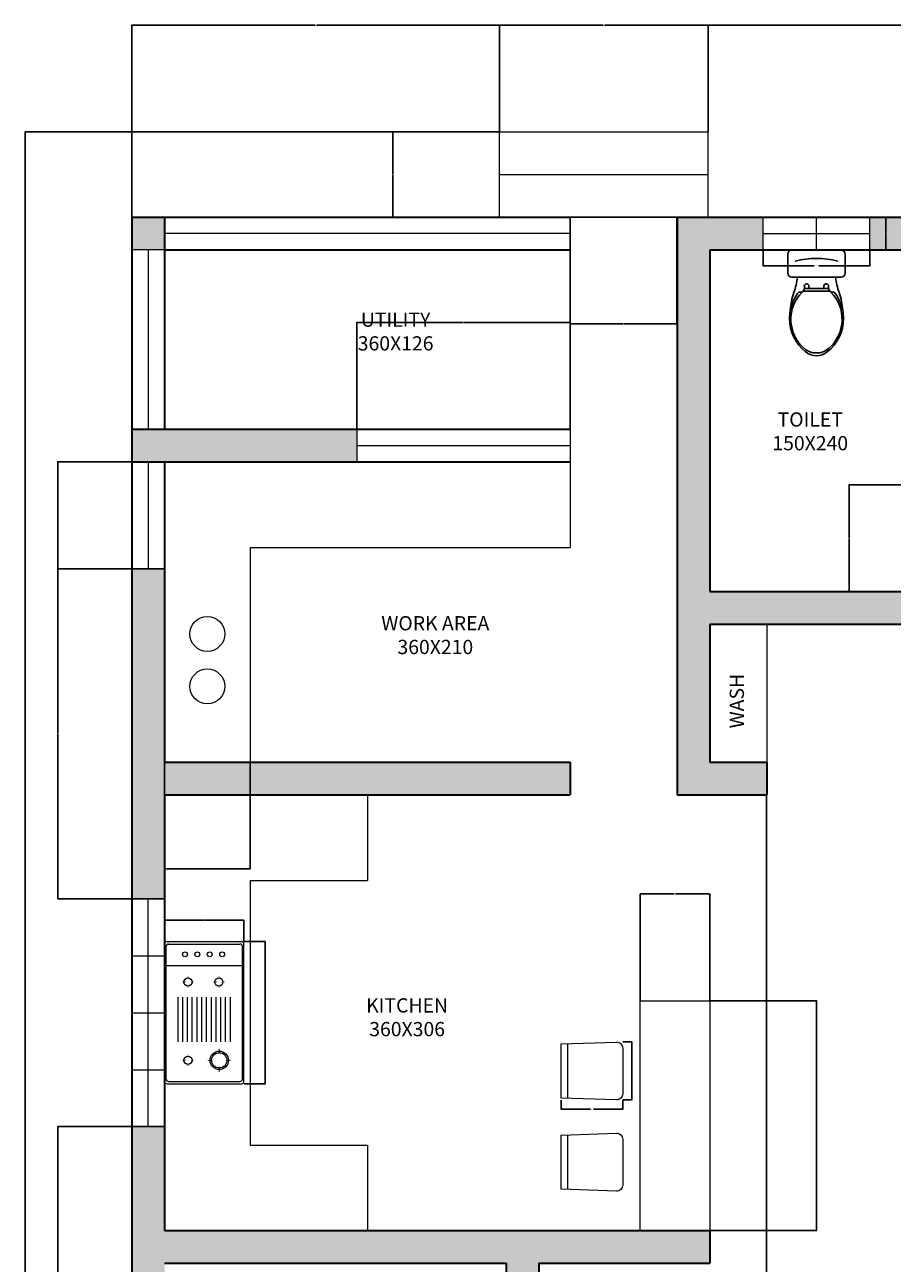
# Model space of a CAD drawing. Units: centimetres. Extents: x 2178 to 3635, y 1064 to 2635.
# Tile 5 of 9: x 2178 to 2788, y 1765 to 2635. Entities that reach past the tile are written whole.
import ezdxf

# ---------------------------------------------------------------- set-up
doc = ezdxf.new("R2010")
doc.units = ezdxf.units.CM
for name, color, linetype, lineweight in [('A-ANNO-DIMS', 2, 'Continuous', 18), ('A-AREA-IDEN', 7, 'Continuous', 18), ('A-DOOR', 32, 'Continuous', 25), ('A-EQPM', 42, 'Continuous', 18), ('A-FLOR-CASE', 32, 'Continuous', 18), ('A-FLOR-FIXT', 42, 'Continuous', 18), ('A-FLOR-STRS', 7, 'Continuous', 18), ('A-FURN', 42, 'Continuous', 18), ('A-GLAZ', 4, 'Continuous', 18), ('A-WALL', 7, 'Continuous', 35)]:
    doc.layers.add(name, color=color, linetype=linetype, lineweight=lineweight)
doc.layers.add('A-WALL-PATT', color=18, linetype='Continuous', lineweight=13, true_color=0x000000)
doc.layers.add('WC-Detail_dwgmodels.com', color=251, linetype='Continuous')
doc.layers.add('WC-Outline_dwgmodels.com', color=250, linetype='Continuous')
doc.styles.get("Standard").update_dxf_attribs({"font": 'arial.ttf'})
doc.dimstyles.get("Standard").update_dxf_attribs({"dimtxt": 0.18, "dimasz": 0.18, "dimexe": 0.18, "dimexo": 0.0625, "dimgap": 0.09, "dimtad": 0, "dimtih": 1, "dimtoh": 1, "dimdec": 4, "dimzin": 0, "dimdsep": 46, "dimtxsty": 'Standard', "dimcen": 0.09, "dimadec": 0, "dimazin": 0, "dimtfac": 1, "dimtdec": 4, "dimtofl": 0, "dimtmove": 0, "dimatfit": 3, "dimfxl": 1, "dimtolj": 1, "dimtzin": 0, "dimarcsym": 0})

# ---------------------------------------------------------------- blocks, each defined once
blk = doc.blocks.new('pan')
at = {"layer": 'WC-Detail_dwgmodels.com'}
for p, q in [((2845.06, 2654.5), (2845.98, 2656.18)), ((2854.51, 2654.5), (2845.06, 2654.5)), ((2845.98, 2656.18), (2845.98, 2658.01)), ((2849.25, 2656.18), (2845.98, 2656.18)), ((2849.25, 2658.01), (2849.25, 2656.18)), ((2854.51, 2656.18), (2849.25, 2656.18)), ((2854.51, 2656.18), (2859.76, 2656.18)), ((2854.51, 2654.5), (2863.95, 2654.5)), ((2859.76, 2658.01), (2859.76, 2656.18)), ((2859.76, 2656.18), (2863.04, 2656.18)), ((2863.04, 2656.18), (2863.04, 2658.01)), ((2863.95, 2654.5), (2863.04, 2656.18)), ((2844.36, 2653.82), (2842.09, 2653.82)), ((2864.65, 2653.82), (2866.93, 2653.82))]:
    blk.add_line(p, q, dxfattribs=at)
for centre, radius, start, end in [((2854.54, 2618.37), 59.08, 90.02796, 104.67123), ((2854.48, 2618.37), 59.08, 75.32877, 89.97204), ((2863.72, 2634.72), 27.2, 133.32364, 135.38283), ((2847.61, 2658.01), 1.64, 0, 180), ((2861.4, 2658.01), 1.64, 0, 180), ((2845.29, 2634.72), 27.2, 44.61717, 46.67636), ((2863.72, 2634.72), 27.2, 135.38283, 229.26806), ((2865.36, 2635.16), 29.83, 141.274, 162.76494), ((2845.29, 2634.72), 27.2, 310.73194, 44.61717), ((2843.66, 2635.16), 29.83, 14.64821, 38.726), ((2865.36, 2635.16), 29.83, 162.76494, 168.85834), ((2843.66, 2635.16), 29.83, 11.14166, 14.64821), ((2854.36, 2623.84), 12.85, 229.26806, 270.66836), ((2854.66, 2623.84), 12.85, 269.33164, 310.73194)]:
    blk.add_arc(centre, radius, start, end, dxfattribs=at)
at = {"layer": 'WC-Outline_dwgmodels.com'}
for p, q in [((2834.37, 2680.53), (2834.37, 2667.05)), ((2854.51, 2683.42), (2837.26, 2683.42)), ((2871.75, 2683.42), (2854.51, 2683.42)), ((2874.65, 2667.05), (2874.65, 2680.53)), ((2837.26, 2664.16), (2841.21, 2664.16)), ((2841.21, 2664.16), (2854.51, 2664.16)), ((2867.8, 2664.16), (2854.51, 2664.16)), ((2867.8, 2664.16), (2871.75, 2664.16))]:
    blk.add_line(p, q, dxfattribs=at)
for centre, radius, start, end in [((2837.26, 2680.53), 2.89, 90, 180), ((2871.75, 2680.53), 2.89, 360, 90), ((2837.26, 2667.05), 2.89, 180, 270), ((2788.54, 2671.16), 53.13, 340.44424, 352.4299), ((2920.47, 2671.16), 53.13, 187.5701, 199.55576), ((2871.75, 2667.05), 2.89, 270, 0), ((2880.9, 2638.36), 44.88, 160.44424, 176.71895), ((2828.12, 2638.36), 44.88, 3.28105, 19.55576), ((2865.36, 2635.16), 29.83, 168.85834, 179.8559), ((2843.66, 2635.16), 29.83, 0.1441, 11.14166), ((2865.36, 2635.16), 29.83, 179.8559, 231.74169), ((2843.66, 2635.16), 29.83, 308.25831, 0.1441), ((2854.51, 2621.4), 12.31, 231.74169, 269.98853), ((2854.5, 2621.4), 12.31, 270.01147, 308.25831)]:
    blk.add_arc(centre, radius, start, end, dxfattribs=at)
blk = doc.blocks.new('cooktop')
for p, q in [((2318.02, 2660.21), (2318.02, 2613.21)), ((2319.52, 2661.71), (2406.13, 2661.71)), ((2319.52, 2659.21), (2319.52, 2614.21)), ((2321.02, 2660.71), (2404.63, 2660.71)), ((2392.56, 2660.71), (2392.56, 2612.71)), ((2406.13, 2659.21), (2406.13, 2614.21)), ((2407.63, 2660.21), (2407.63, 2613.21)), ((2332.64, 2648.75), (2333.04, 2648.75)), ((2344.49, 2653.27), (2372.74, 2653.27)), ((2344.49, 2650.27), (2372.74, 2650.27)), ((2344.49, 2647.27), (2372.74, 2647.27)), ((2382.04, 2648.75), (2382.44, 2648.75)), ((2344.49, 2644.27), (2372.74, 2644.27)), ((2344.49, 2641.27), (2372.74, 2641.27)), ((2344.49, 2638.27), (2372.74, 2638.27)), ((2344.49, 2635.27), (2372.74, 2635.27)), ((2344.49, 2632.27), (2372.74, 2632.27)), ((2344.49, 2629.27), (2372.74, 2629.27)), ((2344.49, 2626.27), (2372.74, 2626.27)), ((2344.49, 2623.27), (2372.74, 2623.27)), ((2382.04, 2629.31), (2382.44, 2629.31)), ((2344.49, 2620.27), (2372.74, 2620.27)), ((2319.52, 2611.71), (2406.13, 2611.71)), ((2321.02, 2612.71), (2404.63, 2612.71))]:
    blk.add_line(p, q)
for centre, radius in [((2332.84, 2646.95), 2.58), ((2382.24, 2646.95), 2.58), ((2399.61, 2648.89), 1.53), ((2399.61, 2641.09), 1.53), ((2332.84, 2627.26), 5.81), ((2332.84, 2627.26), 4.81), ((2399.61, 2633.28), 1.53), ((2382.24, 2627.51), 2.58), ((2399.61, 2625.48), 1.53)]:
    blk.add_circle(centre, radius)
for centre, start, end in [((2319.52, 2660.21), 90, 180), ((2321.02, 2659.21), 90, 180), ((2404.63, 2659.21), 0, 90), ((2406.13, 2660.21), 0, 90), ((2319.52, 2613.21), 180, 270), ((2321.02, 2614.21), 180, 270), ((2404.63, 2614.21), 270, 0), ((2406.13, 2613.21), 270, 0)]:
    blk.add_arc(centre, 1.5, start, end)
for points in [[(2329.26, 2646.75), (2329.26, 2647.15), (2331.04, 2646.75), (2331.04, 2647.15)], [(2332.64, 2650.53), (2333.04, 2650.53), (2332.64, 2648.75), (2333.04, 2648.75)], [(2336.42, 2647.15), (2336.42, 2646.75), (2334.64, 2647.15), (2334.64, 2646.75)], [(2378.66, 2646.75), (2378.66, 2647.15), (2380.44, 2646.75), (2380.44, 2647.15)], [(2382.04, 2650.53), (2382.44, 2650.53), (2382.04, 2648.75), (2382.44, 2648.75)], [(2385.82, 2647.15), (2385.82, 2646.75), (2384.04, 2647.15), (2384.04, 2646.75)], [(2333.04, 2643.37), (2332.64, 2643.37), (2333.04, 2645.14), (2332.64, 2645.14)], [(2382.44, 2643.37), (2382.04, 2643.37), (2382.44, 2645.14), (2382.04, 2645.14)], [(2332.54, 2634.56), (2333.14, 2634.56), (2332.54, 2631.56), (2333.14, 2631.56)], [(2382.04, 2631.09), (2382.44, 2631.09), (2382.04, 2629.31), (2382.44, 2629.31)], [(2325.54, 2626.96), (2325.54, 2627.56), (2328.54, 2626.96), (2328.54, 2627.56)], [(2333.14, 2619.95), (2332.54, 2619.95), (2333.14, 2622.96), (2332.54, 2622.96)], [(2340.15, 2627.56), (2340.15, 2626.96), (2337.14, 2627.56), (2337.14, 2626.96)], [(2378.66, 2627.31), (2378.66, 2627.71), (2380.44, 2627.31), (2380.44, 2627.71)], [(2382.44, 2623.93), (2382.04, 2623.93), (2382.44, 2625.71), (2382.04, 2625.71)], [(2385.82, 2627.71), (2385.82, 2627.31), (2384.04, 2627.71), (2384.04, 2627.31)]]:
    blk.add_solid(points)
blk = doc.blocks.new('c')
blk.add_lwpolyline([(3808.85, 1833.77), (3776.18, 1834.86), (3776.18, 1867.04), (3808.85, 1868.12, -0.424007), (3812.61, 1864.48), (3812.61, 1837.41, -0.424007)], format="xyb", close=True)
blk.add_lwpolyline([(3779.83, 1867.16), (3779.83, 1834.74)])
blk = doc.blocks.new('WIN-1600-4LT')
for p, q in [((0, 23), (0, 0)), ((40, 23), (40, 0)), ((80, 23), (80, 0)), ((120, 23), (120, 0)), ((160, 23), (160, 0)), ((0, 11.5), (160, 11.5))]:
    blk.add_line(p, q)
blk = doc.blocks.new('WIN-0750-2LT')
for p, q in [((0, 0), (0, 23)), ((37.5, 0), (37.5, 23)), ((75, 0), (75, 23)), ((0, 11.5), (75, 11.5))]:
    blk.add_line(p, q)
blk = doc.blocks.new('DOOR-0750')
blk.add_line((0, 0), (75, 0))
blk = doc.blocks.new('*D22')
at = {"layer": 'A-ANNO-DIMS', "color": 0, "lineweight": -2, "transparency": 16777216}
for p, q in [((2555.32, 1879.23), (2555.32, 1872.64)), ((2555.5, 1872.82), (2575.93, 1872.82)), ((2598.28, 1872.82), (2577.84, 1872.82)), ((2598.46, 1879.23), (2598.46, 1872.64))]:
    blk.add_line(p, q, dxfattribs=at)
at = {"layer": 'A-ANNO-DIMS', "color": 0, "transparency": 16777216}
for points in [[(2555.5, 1872.85), (2555.5, 1872.79), (2555.32, 1872.82)], [(2598.28, 1872.85), (2598.28, 1872.79), (2598.46, 1872.82)]]:
    blk.add_solid(points, dxfattribs=at)
at = {"layer": 'Defpoints', "color": 0, "transparency": 16777216}
for p in [(2555.32, 1879.29), (2598.46, 1879.29), (2598.46, 1872.82)]:
    blk.add_point(p, dxfattribs=at)
at = {"layer": 'A-ANNO-DIMS', "color": 0, "transparency": 16777216, "insert": (2576.89, 1872.82), "char_height": 0.18, "attachment_point": 5}
blk.add_mtext('\\A1;CHAIR 43 TYP.', dxfattribs=at)
blk = doc.blocks.new('*D23')
at = {"layer": 'A-ANNO-DIMS', "color": 0, "lineweight": -2, "transparency": 16777216}
for p, q in [((2598.52, 1920.05), (2605.11, 1920.05)), ((2604.93, 1919.87), (2604.93, 1899.85)), ((2604.93, 1879.47), (2604.93, 1899.49)), ((2598.52, 1879.29), (2605.11, 1879.29))]:
    blk.add_line(p, q, dxfattribs=at)
at = {"layer": 'A-ANNO-DIMS', "color": 0, "transparency": 16777216}
for points in [[(2604.9, 1919.87), (2604.96, 1919.87), (2604.93, 1920.05)], [(2604.9, 1879.47), (2604.96, 1879.47), (2604.93, 1879.29)]]:
    blk.add_solid(points, dxfattribs=at)
at = {"layer": 'Defpoints', "color": 0, "transparency": 16777216}
for p in [(2598.46, 1920.05), (2604.93, 1920.05), (2598.46, 1879.29)]:
    blk.add_point(p, dxfattribs=at)
at = {"layer": 'A-ANNO-DIMS', "color": 0, "transparency": 16777216, "insert": (2604.93, 1899.67), "char_height": 0.18, "attachment_point": 5}
blk.add_mtext('\\A1;41 TYP.', dxfattribs=at)
blk = doc.blocks.new('*D32')
at = {"layer": 'A-ANNO-DIMS', "color": 0, "lineweight": -2, "transparency": 16777216}
for p, q in [((2697.1, 2476.53), (2697.1, 2465.16)), ((2772.1, 2476.53), (2772.1, 2465.16)), ((2697.28, 2465.34), (2732.97, 2465.34)), ((2771.92, 2465.34), (2736.24, 2465.34))]:
    blk.add_line(p, q, dxfattribs=at)
at = {"layer": 'A-ANNO-DIMS', "color": 0, "transparency": 16777216}
for points in [[(2697.28, 2465.37), (2697.28, 2465.31), (2697.1, 2465.34)], [(2771.92, 2465.37), (2771.92, 2465.31), (2772.1, 2465.34)]]:
    blk.add_solid(points, dxfattribs=at)
at = {"layer": 'Defpoints', "color": 0, "transparency": 16777216}
for p in [(2697.1, 2476.59), (2772.1, 2476.59), (2772.1, 2465.34)]:
    blk.add_point(p, dxfattribs=at)
at = {"layer": 'A-ANNO-DIMS', "color": 0, "transparency": 16777216, "insert": (2734.6, 2465.34), "char_height": 0.18, "attachment_point": 5}
blk.add_mtext('\\A1;2-LIGHT WINDOW 75 TYP.', dxfattribs=at)
blk = doc.blocks.new('*D33')
at = {"layer": 'A-ANNO-DIMS', "color": 0, "lineweight": -2, "transparency": 16777216}
for p, q in [((2772.17, 2499.59), (2783.53, 2499.59)), ((2783.35, 2499.41), (2783.35, 2488.27)), ((2783.35, 2476.77), (2783.35, 2487.91)), ((2772.17, 2476.59), (2783.53, 2476.59))]:
    blk.add_line(p, q, dxfattribs=at)
at = {"layer": 'A-ANNO-DIMS', "color": 0, "transparency": 16777216}
for points in [[(2783.32, 2499.41), (2783.38, 2499.41), (2783.35, 2499.59)], [(2783.32, 2476.77), (2783.38, 2476.77), (2783.35, 2476.59)]]:
    blk.add_solid(points, dxfattribs=at)
at = {"layer": 'Defpoints', "color": 0, "transparency": 16777216}
for p in [(2772.1, 2499.59), (2783.35, 2499.59), (2772.1, 2476.59)]:
    blk.add_point(p, dxfattribs=at)
at = {"layer": 'A-ANNO-DIMS', "color": 0, "transparency": 16777216, "insert": (2783.35, 2488.09), "char_height": 0.18, "attachment_point": 5}
blk.add_mtext('\\A1;23 TYP.', dxfattribs=at)
blk = doc.blocks.new('*D44')
at = {"layer": 'A-ANNO-DIMS', "color": 0, "lineweight": -2, "transparency": 16777216}
for p, q in [((2332.41, 1990.54), (2347.51, 1990.54)), ((2347.33, 1990.36), (2347.33, 1940.77)), ((2347.33, 1890.82), (2347.33, 1940.41)), ((2332.41, 1890.64), (2347.51, 1890.64))]:
    blk.add_line(p, q, dxfattribs=at)
at = {"layer": 'A-ANNO-DIMS', "color": 0, "transparency": 16777216}
for points in [[(2347.3, 1990.36), (2347.36, 1990.36), (2347.33, 1990.54)], [(2347.3, 1890.82), (2347.36, 1890.82), (2347.33, 1890.64)]]:
    blk.add_solid(points, dxfattribs=at)
at = {"layer": 'Defpoints', "color": 0, "transparency": 16777216}
for p in [(2332.35, 1990.54), (2347.33, 1990.54), (2332.35, 1890.64)]:
    blk.add_point(p, dxfattribs=at)
at = {"layer": 'A-ANNO-DIMS', "color": 0, "transparency": 16777216, "insert": (2347.33, 1940.59), "char_height": 0.18, "attachment_point": 5}
blk.add_mtext('\\A1;COOKTOP 100', dxfattribs=at)
blk = doc.blocks.new('*D45')
at = {"layer": 'A-ANNO-DIMS', "color": 0, "lineweight": -2, "transparency": 16777216}
for p, q in [((2276.6, 1990.6), (2276.6, 2005.7)), ((2276.78, 2005.52), (2304.26, 2005.52)), ((2332.17, 2005.52), (2304.69, 2005.52)), ((2332.35, 1990.6), (2332.35, 2005.7))]:
    blk.add_line(p, q, dxfattribs=at)
at = {"layer": 'A-ANNO-DIMS', "color": 0, "transparency": 16777216}
for points in [[(2276.78, 2005.55), (2276.78, 2005.49), (2276.6, 2005.52)], [(2332.17, 2005.55), (2332.17, 2005.49), (2332.35, 2005.52)]]:
    blk.add_solid(points, dxfattribs=at)
at = {"layer": 'Defpoints', "color": 0, "transparency": 16777216}
for p in [(2276.6, 2005.52), (2276.6, 1990.54), (2332.35, 1990.54)]:
    blk.add_point(p, dxfattribs=at)
at = {"layer": 'A-ANNO-DIMS', "color": 0, "transparency": 16777216, "insert": (2304.47, 2005.52), "char_height": 0.18, "attachment_point": 5}
blk.add_mtext('\\A1;56', dxfattribs=at)
blk = doc.blocks.new('*D47')
at = {"layer": 'A-ANNO-DIMS', "color": 0, "lineweight": -2, "transparency": 16777216}
for p, q in [((2511.88, 2559.59), (2178.42, 2559.59)), ((2178.6, 2559.41), (2178.6, 1874.27)), ((2178.6, 1188.77), (2178.6, 1873.91)), ((2253.54, 1188.59), (2178.42, 1188.59))]:
    blk.add_line(p, q, dxfattribs=at)
at = {"layer": 'A-ANNO-DIMS', "color": 0, "transparency": 16777216}
for points in [[(2178.57, 2559.41), (2178.63, 2559.41), (2178.6, 2559.59)], [(2178.57, 1188.77), (2178.63, 1188.77), (2178.6, 1188.59)]]:
    blk.add_solid(points, dxfattribs=at)
at = {"layer": 'Defpoints', "color": 0, "transparency": 16777216}
for p in [(2178.6, 2559.59), (2511.95, 2559.59), (2253.6, 1188.59)]:
    blk.add_point(p, dxfattribs=at)
at = {"layer": 'A-ANNO-DIMS', "color": 0, "transparency": 16777216, "insert": (2178.6, 1874.09), "char_height": 0.18, "attachment_point": 5}
blk.add_mtext('\\A1;1371', dxfattribs=at)
blk = doc.blocks.new('*D48')
at = {"layer": 'A-ANNO-DIMS', "color": 0, "lineweight": -2, "transparency": 16777216}
for p, q in [((2253.6, 2499.65), (2253.6, 2634.77)), ((2253.78, 2634.59), (2382.31, 2634.59)), ((2511.77, 2634.59), (2383.24, 2634.59)), ((2511.95, 2559.65), (2511.95, 2634.77))]:
    blk.add_line(p, q, dxfattribs=at)
at = {"layer": 'A-ANNO-DIMS', "color": 0, "transparency": 16777216}
for points in [[(2253.78, 2634.62), (2253.78, 2634.56), (2253.6, 2634.59)], [(2511.77, 2634.62), (2511.77, 2634.56), (2511.95, 2634.59)]]:
    blk.add_solid(points, dxfattribs=at)
at = {"layer": 'Defpoints', "color": 0, "transparency": 16777216}
for p in [(2511.95, 2634.59), (2511.95, 2559.59), (2253.6, 2499.59)]:
    blk.add_point(p, dxfattribs=at)
at = {"layer": 'A-ANNO-DIMS', "color": 0, "transparency": 16777216, "insert": (2382.78, 2634.59), "char_height": 0.18, "attachment_point": 5}
blk.add_mtext('\\A1;258.34', dxfattribs=at)
blk = doc.blocks.new('*D49')
at = {"layer": 'A-ANNO-DIMS', "color": 0, "lineweight": -2, "transparency": 16777216}
for p, q in [((2511.95, 2559.65), (2511.95, 2634.77)), ((2512.13, 2634.59), (2584.8, 2634.59)), ((2658.38, 2634.59), (2585.71, 2634.59)), ((2658.56, 2559.65), (2658.56, 2634.77))]:
    blk.add_line(p, q, dxfattribs=at)
at = {"layer": 'A-ANNO-DIMS', "color": 0, "transparency": 16777216}
for points in [[(2512.13, 2634.62), (2512.13, 2634.56), (2511.95, 2634.59)], [(2658.38, 2634.62), (2658.38, 2634.56), (2658.56, 2634.59)]]:
    blk.add_solid(points, dxfattribs=at)
at = {"layer": 'Defpoints', "color": 0, "transparency": 16777216}
for p in [(2658.56, 2634.59), (2511.95, 2559.59), (2658.56, 2559.59)]:
    blk.add_point(p, dxfattribs=at)
at = {"layer": 'A-ANNO-DIMS', "color": 0, "transparency": 16777216, "insert": (2585.25, 2634.59), "char_height": 0.18, "attachment_point": 5}
blk.add_mtext('\\A1;146.62', dxfattribs=at)
blk = doc.blocks.new('*D50')
at = {"layer": 'A-ANNO-DIMS', "color": 0, "lineweight": -2, "transparency": 16777216}
for p, q in [((2658.56, 2559.65), (2658.56, 2634.77)), ((2658.74, 2634.59), (2926.79, 2634.59)), ((3195.42, 2634.59), (2927.37, 2634.59)), ((3195.6, 2499.65), (3195.6, 2634.77))]:
    blk.add_line(p, q, dxfattribs=at)
at = {"layer": 'A-ANNO-DIMS', "color": 0, "transparency": 16777216}
for points in [[(2658.74, 2634.62), (2658.74, 2634.56), (2658.56, 2634.59)], [(3195.42, 2634.62), (3195.42, 2634.56), (3195.6, 2634.59)]]:
    blk.add_solid(points, dxfattribs=at)
at = {"layer": 'Defpoints', "color": 0, "transparency": 16777216}
for p in [(3195.6, 2634.59), (2658.56, 2559.59), (3195.6, 2499.59)]:
    blk.add_point(p, dxfattribs=at)
at = {"layer": 'A-ANNO-DIMS', "color": 0, "transparency": 16777216, "insert": (2927.08, 2634.59), "char_height": 0.18, "attachment_point": 5}
blk.add_mtext('\\A1;537', dxfattribs=at)
blk = doc.blocks.new('*D52')
at = {"layer": 'A-ANNO-DIMS', "color": 0, "lineweight": -2, "transparency": 16777216}
for p, q in [((2511.88, 2559.59), (2436.77, 2559.59)), ((2436.95, 2559.41), (2436.95, 2529.77)), ((2436.95, 2499.77), (2436.95, 2529.41)), ((2511.88, 2499.59), (2436.77, 2499.59))]:
    blk.add_line(p, q, dxfattribs=at)
at = {"layer": 'A-ANNO-DIMS', "color": 0, "transparency": 16777216}
for points in [[(2436.92, 2559.41), (2436.98, 2559.41), (2436.95, 2559.59)], [(2436.92, 2499.77), (2436.98, 2499.77), (2436.95, 2499.59)]]:
    blk.add_solid(points, dxfattribs=at)
at = {"layer": 'Defpoints', "color": 0, "transparency": 16777216}
for p in [(2436.95, 2559.59), (2511.95, 2559.59), (2511.95, 2499.59)]:
    blk.add_point(p, dxfattribs=at)
at = {"layer": 'A-ANNO-DIMS', "color": 0, "transparency": 16777216, "insert": (2436.95, 2529.59), "char_height": 0.18, "attachment_point": 5}
blk.add_mtext('\\A1;60', dxfattribs=at)
blk = doc.blocks.new('*D63')
at = {"layer": 'A-ANNO-DIMS', "color": 0, "lineweight": -2, "transparency": 16777216}
for p, q in [((2699.6, 2093.53), (2699.6, 1113.41)), ((2809.6, 2093.53), (2809.6, 1113.41)), ((2699.78, 1113.59), (2754.32, 1113.59)), ((2809.42, 1113.59), (2754.88, 1113.59))]:
    blk.add_line(p, q, dxfattribs=at)
at = {"layer": 'A-ANNO-DIMS', "color": 0, "transparency": 16777216}
for points in [[(2699.78, 1113.62), (2699.78, 1113.56), (2699.6, 1113.59)], [(2809.42, 1113.62), (2809.42, 1113.56), (2809.6, 1113.59)]]:
    blk.add_solid(points, dxfattribs=at)
at = {"layer": 'Defpoints', "color": 0, "transparency": 16777216}
for p in [(2699.6, 2093.59), (2809.6, 2093.59), (2809.6, 1113.59)]:
    blk.add_point(p, dxfattribs=at)
at = {"layer": 'A-ANNO-DIMS', "color": 0, "transparency": 16777216, "insert": (2754.6, 1113.59), "char_height": 0.18, "attachment_point": 5}
blk.add_mtext('\\A1;110', dxfattribs=at)
blk = doc.blocks.new('*D64')
at = {"layer": 'A-ANNO-DIMS', "color": 0, "lineweight": -2, "transparency": 16777216}
for p, q in [((2561.6, 2499.53), (2561.6, 2424.41)), ((2636.6, 2499.53), (2636.6, 2424.41)), ((2561.78, 2424.59), (2598.89, 2424.59)), ((2636.42, 2424.59), (2599.32, 2424.59))]:
    blk.add_line(p, q, dxfattribs=at)
at = {"layer": 'A-ANNO-DIMS', "color": 0, "transparency": 16777216}
for points in [[(2561.78, 2424.62), (2561.78, 2424.56), (2561.6, 2424.59)], [(2636.42, 2424.62), (2636.42, 2424.56), (2636.6, 2424.59)]]:
    blk.add_solid(points, dxfattribs=at)
at = {"layer": 'Defpoints', "color": 0, "transparency": 16777216}
for p in [(2561.6, 2499.59), (2636.6, 2499.59), (2561.6, 2424.59)]:
    blk.add_point(p, dxfattribs=at)
at = {"layer": 'A-ANNO-DIMS', "color": 0, "transparency": 16777216, "insert": (2599.1, 2424.59), "char_height": 0.18, "attachment_point": 5}
blk.add_mtext('\\A1;75', dxfattribs=at)
blk = doc.blocks.new('*D66')
at = {"layer": 'A-ANNO-DIMS', "color": 0, "lineweight": -2, "transparency": 16777216}
for p, q in [((2832.54, 2311.59), (2757.42, 2311.59)), ((2757.6, 2311.41), (2757.6, 2274.27)), ((2757.6, 2236.77), (2757.6, 2273.91)), ((2832.54, 2236.59), (2757.42, 2236.59))]:
    blk.add_line(p, q, dxfattribs=at)
at = {"layer": 'A-ANNO-DIMS', "color": 0, "transparency": 16777216}
for points in [[(2757.57, 2311.41), (2757.63, 2311.41), (2757.6, 2311.59)], [(2757.57, 2236.77), (2757.63, 2236.77), (2757.6, 2236.59)]]:
    blk.add_solid(points, dxfattribs=at)
at = {"layer": 'Defpoints', "color": 0, "transparency": 16777216}
for p in [(2757.6, 2311.59), (2832.6, 2311.59), (2832.6, 2236.59)]:
    blk.add_point(p, dxfattribs=at)
at = {"layer": 'A-ANNO-DIMS', "color": 0, "transparency": 16777216, "insert": (2757.6, 2274.09), "char_height": 0.18, "attachment_point": 5}
blk.add_mtext('\\A1;75', dxfattribs=at)
blk = doc.blocks.new('*D72')
at = {"layer": 'A-ANNO-DIMS', "color": 0, "lineweight": -2, "transparency": 16777216}
for p, q in [((2276.54, 1860.59), (2201.42, 1860.59)), ((2201.6, 1860.41), (2201.6, 1796.52)), ((2201.6, 1732.27), (2201.6, 1796.16)), ((2276.54, 1732.09), (2201.42, 1732.09))]:
    blk.add_line(p, q, dxfattribs=at)
at = {"layer": 'A-ANNO-DIMS', "color": 0, "transparency": 16777216}
for points in [[(2201.57, 1860.41), (2201.63, 1860.41), (2201.6, 1860.59)], [(2201.57, 1732.27), (2201.63, 1732.27), (2201.6, 1732.09)]]:
    blk.add_solid(points, dxfattribs=at)
at = {"layer": 'Defpoints', "color": 0, "transparency": 16777216}
for p in [(2201.6, 1860.59), (2276.6, 1860.59), (2276.6, 1732.09)]:
    blk.add_point(p, dxfattribs=at)
at = {"layer": 'A-ANNO-DIMS', "color": 0, "transparency": 16777216, "insert": (2201.6, 1796.34), "char_height": 0.18, "attachment_point": 5}
blk.add_mtext('\\A1;128.5', dxfattribs=at)
blk = doc.blocks.new('*D73')
at = {"layer": 'A-ANNO-DIMS', "color": 0, "lineweight": -2, "transparency": 16777216}
for p, q in [((2276.54, 2252.59), (2201.42, 2252.59)), ((2201.6, 2252.41), (2201.6, 2136.77)), ((2201.6, 2020.77), (2201.6, 2136.41)), ((2276.54, 2020.59), (2201.42, 2020.59))]:
    blk.add_line(p, q, dxfattribs=at)
at = {"layer": 'A-ANNO-DIMS', "color": 0, "transparency": 16777216}
for points in [[(2201.57, 2252.41), (2201.63, 2252.41), (2201.6, 2252.59)], [(2201.57, 2020.77), (2201.63, 2020.77), (2201.6, 2020.59)]]:
    blk.add_solid(points, dxfattribs=at)
at = {"layer": 'Defpoints', "color": 0, "transparency": 16777216}
for p in [(2201.6, 2252.59), (2276.6, 2252.59), (2276.6, 2020.59)]:
    blk.add_point(p, dxfattribs=at)
at = {"layer": 'A-ANNO-DIMS', "color": 0, "transparency": 16777216, "insert": (2201.6, 2136.59), "char_height": 0.18, "attachment_point": 5}
blk.add_mtext('\\A1;232', dxfattribs=at)
blk = doc.blocks.new('*D74')
at = {"layer": 'A-ANNO-DIMS', "color": 0, "lineweight": -2, "transparency": 16777216}
for p, q in [((2276.54, 2327.59), (2201.42, 2327.59)), ((2201.6, 2327.41), (2201.6, 2290.27)), ((2201.6, 2252.77), (2201.6, 2289.91)), ((2276.54, 2252.59), (2201.42, 2252.59))]:
    blk.add_line(p, q, dxfattribs=at)
at = {"layer": 'A-ANNO-DIMS', "color": 0, "transparency": 16777216}
for points in [[(2201.57, 2327.41), (2201.63, 2327.41), (2201.6, 2327.59)], [(2201.57, 2252.77), (2201.63, 2252.77), (2201.6, 2252.59)]]:
    blk.add_solid(points, dxfattribs=at)
at = {"layer": 'Defpoints', "color": 0, "transparency": 16777216}
for p in [(2201.6, 2327.59), (2276.6, 2327.59), (2276.6, 2252.59)]:
    blk.add_point(p, dxfattribs=at)
at = {"layer": 'A-ANNO-DIMS', "color": 0, "transparency": 16777216, "insert": (2201.6, 2290.09), "char_height": 0.18, "attachment_point": 5}
blk.add_mtext('\\A1;75', dxfattribs=at)
blk = doc.blocks.new('*D81')
at = {"layer": 'A-ANNO-DIMS', "color": 0, "lineweight": -2, "transparency": 16777216}
for p, q in [((2276.6, 2116.53), (2276.6, 2041.41)), ((2336.6, 2116.53), (2336.6, 2041.41)), ((2276.78, 2041.59), (2306.39, 2041.59)), ((2336.42, 2041.59), (2306.82, 2041.59))]:
    blk.add_line(p, q, dxfattribs=at)
at = {"layer": 'A-ANNO-DIMS', "color": 0, "transparency": 16777216}
for points in [[(2276.78, 2041.62), (2276.78, 2041.56), (2276.6, 2041.59)], [(2336.42, 2041.62), (2336.42, 2041.56), (2336.6, 2041.59)]]:
    blk.add_solid(points, dxfattribs=at)
at = {"layer": 'Defpoints', "color": 0, "transparency": 16777216}
for p in [(2276.6, 2116.59), (2336.6, 2116.59), (2276.6, 2041.59)]:
    blk.add_point(p, dxfattribs=at)
at = {"layer": 'A-ANNO-DIMS', "color": 0, "transparency": 16777216, "insert": (2306.6, 2041.59), "char_height": 0.18, "attachment_point": 5}
blk.add_mtext('\\A1;60', dxfattribs=at)
blk = doc.blocks.new('*D82')
at = {"layer": 'A-ANNO-DIMS', "color": 0, "lineweight": -2, "transparency": 16777216}
for p, q in [((2411.6, 2350.65), (2411.6, 2425.77)), ((2411.78, 2425.59), (2486.32, 2425.59)), ((2561.42, 2425.59), (2486.88, 2425.59)), ((2561.6, 2350.65), (2561.6, 2425.77))]:
    blk.add_line(p, q, dxfattribs=at)
at = {"layer": 'A-ANNO-DIMS', "color": 0, "transparency": 16777216}
for points in [[(2411.78, 2425.62), (2411.78, 2425.56), (2411.6, 2425.59)], [(2561.42, 2425.62), (2561.42, 2425.56), (2561.6, 2425.59)]]:
    blk.add_solid(points, dxfattribs=at)
at = {"layer": 'Defpoints', "color": 0, "transparency": 16777216}
for p in [(2561.6, 2425.59), (2411.6, 2350.59), (2561.6, 2350.59)]:
    blk.add_point(p, dxfattribs=at)
at = {"layer": 'A-ANNO-DIMS', "color": 0, "transparency": 16777216, "insert": (2486.6, 2425.59), "char_height": 0.18, "attachment_point": 5}
blk.add_mtext('\\A1;150', dxfattribs=at)
blk = doc.blocks.new('*D83')
at = {"layer": 'A-ANNO-DIMS', "color": 0, "lineweight": -2, "transparency": 16777216}
for p, q in [((2610.62, 1949.1), (2610.62, 2024.22)), ((2610.8, 2024.04), (2634.71, 2024.04)), ((2659.42, 2024.04), (2635.51, 2024.04)), ((2659.6, 1949.1), (2659.6, 2024.22))]:
    blk.add_line(p, q, dxfattribs=at)
at = {"layer": 'A-ANNO-DIMS', "color": 0, "transparency": 16777216}
for points in [[(2610.8, 2024.07), (2610.8, 2024.01), (2610.62, 2024.04)], [(2659.42, 2024.07), (2659.42, 2024.01), (2659.6, 2024.04)]]:
    blk.add_solid(points, dxfattribs=at)
at = {"layer": 'Defpoints', "color": 0, "transparency": 16777216}
for p in [(2659.6, 2024.04), (2610.62, 1949.04), (2659.6, 1949.04)]:
    blk.add_point(p, dxfattribs=at)
at = {"layer": 'A-ANNO-DIMS', "color": 0, "transparency": 16777216, "insert": (2635.11, 2024.04), "char_height": 0.18, "attachment_point": 5}
blk.add_mtext('\\A1;48.99', dxfattribs=at)
blk = doc.blocks.new('*D84')
at = {"layer": 'A-ANNO-DIMS', "color": 0, "lineweight": -2, "transparency": 16777216}
for p, q in [((2659.67, 1949.04), (2734.78, 1949.04)), ((2734.6, 1948.86), (2734.6, 1868.5)), ((2734.6, 1787.77), (2734.6, 1868.13)), ((2659.67, 1787.59), (2734.78, 1787.59))]:
    blk.add_line(p, q, dxfattribs=at)
at = {"layer": 'A-ANNO-DIMS', "color": 0, "transparency": 16777216}
for points in [[(2734.57, 1948.86), (2734.63, 1948.86), (2734.6, 1949.04)], [(2734.57, 1787.77), (2734.63, 1787.77), (2734.6, 1787.59)]]:
    blk.add_solid(points, dxfattribs=at)
at = {"layer": 'Defpoints', "color": 0, "transparency": 16777216}
for p in [(2659.6, 1949.04), (2659.6, 1787.59), (2734.6, 1787.59)]:
    blk.add_point(p, dxfattribs=at)
at = {"layer": 'A-ANNO-DIMS', "color": 0, "transparency": 16777216, "insert": (2734.6, 1868.31), "char_height": 0.18, "attachment_point": 5}
blk.add_mtext('\\A1;161.45', dxfattribs=at)

msp = doc.modelspace()

# ---------------------------------------------------------------- hatches: boundary and pattern name
at = {"layer": 'A-WALL-PATT'}
h = msp.add_hatch(color=256, dxfattribs=at)
h.dxf.hatch_style = 1
h.paths.add_polyline_path([(2276.605, 2499.59), (2253.605, 2499.59), (2253.605, 2476.59), (2276.605, 2476.59)])
h.paths.add_polyline_path([(2411.605, 2350.59), (2253.605, 2350.59), (2253.605, 2327.59), (2411.605, 2327.59)])
h.paths.add_polyline_path([(2276.605, 2252.59), (2253.605, 2252.59), (2253.605, 2020.59), (2276.605, 2020.59), (2276.605, 2093.59), (2561.605, 2093.59), (2561.605, 2116.59), (2276.605, 2116.59)])
h.paths.add_polyline_path([(2659.605, 1787.59), (2610.616, 1787.59), (2276.605, 1787.59), (2276.605, 1860.59), (2253.605, 1860.59), (2253.605, 1732.09), (2276.605, 1732.09), (2276.605, 1764.59), (2516.605, 1764.59), (2516.605, 1699.59), (2539.605, 1699.59), (2539.605, 1764.59), (2659.605, 1764.59)])
h.paths.add_polyline_path([(2539.605, 1624.59), (2276.605, 1624.59), (2276.605, 1657.09), (2253.605, 1657.09), (2253.605, 1561.59), (2276.605, 1561.59), (2276.605, 1601.59), (2539.605, 1601.59)])
h.paths.add_polyline_path([(2276.605, 1501.59), (2253.605, 1501.59), (2253.605, 1371.59), (2276.605, 1371.59)])
h.paths.add_polyline_path([(2376.605, 1271.59), (2276.605, 1271.59), (2276.605, 1311.59), (2253.605, 1311.59), (2253.605, 1248.59), (2376.605, 1248.59)])
h.paths.add_polyline_path([(2636.605, 1271.59), (2536.605, 1271.59), (2536.605, 1248.59), (2636.605, 1248.59)])
h.paths.add_polyline_path([(2659.605, 1600.59), (2919.605, 1600.59), (2919.605, 1623.59), (2636.605, 1623.59), (2636.605, 1188.59), (2659.605, 1188.59)])
h.paths.add_polyline_path([(2939.605, 1211.59), (2759.605, 1211.59), (2759.605, 1188.59), (2939.605, 1188.59)])
h.paths.add_polyline_path([(3062.605, 1288.59), (3039.605, 1288.59), (3039.605, 1188.59), (3062.605, 1188.59)])
h.paths.add_polyline_path([(3372.605, 1248.59), (3062.605, 1248.59), (3062.605, 1218.59), (3372.605, 1218.59)])
h.paths.add_polyline_path([(3395.605, 1271.59), (3372.605, 1271.59), (3372.605, 1248.59), (3395.605, 1248.59)])
h.paths.add_polyline_path([(3559.605, 1271.59), (3536.605, 1271.59), (3536.605, 1248.59), (3559.605, 1248.59)])
h.paths.add_polyline_path([(3559.605, 1623.59), (3536.605, 1623.59), (3536.605, 1600.59), (3559.605, 1600.59)])
h.paths.add_polyline_path([(3395.605, 1623.59), (3162.605, 1623.59), (3162.605, 1600.59), (3395.605, 1600.59)])
h.paths.add_polyline_path([(3395.605, 1411.59), (3277.1, 1411.59), (3277.1, 1388.59), (3395.605, 1388.59)])
h.paths.add_polyline_path([(3157.1, 1411.59), (3062.605, 1411.59), (3062.605, 1623.59), (3039.605, 1623.59), (3039.605, 1388.59), (3157.1, 1388.59)])
h.paths.add_polyline_path([(3559.605, 1797.09), (3536.605, 1797.09), (3536.605, 1764.59), (3316.605, 1764.59), (3316.605, 1927.59), (3293.605, 1927.59), (3293.605, 1741.59), (3372.605, 1741.59), (3395.605, 1741.59), (3559.605, 1741.59)])
h.paths.add_polyline_path([(3559.605, 1990.59), (3536.605, 1990.59), (3536.605, 1974.446), (3536.605, 1927.59), (3391.605, 1927.59), (3391.605, 1904.59), (3536.605, 1904.59), (3536.605, 1872.09), (3559.605, 1872.09)])
h.paths.add_polyline_path([(3559.605, 2180.59), (3536.605, 2180.59), (3536.605, 2050.59), (3559.605, 2050.59)])
h.paths.add_polyline_path([(3559.605, 2326.59), (3446.105, 2326.59), (3446.105, 2303.59), (3536.605, 2303.59), (3536.605, 2240.59), (3559.605, 2240.59)])
h.paths.add_polyline_path([(3286.105, 2326.59), (3195.605, 2326.59), (3195.605, 2499.59), (3082.605, 2499.59), (3082.605, 2476.59), (3172.605, 2476.59), (3172.605, 2116.59), (2809.605, 2116.59), (2809.605, 2093.59), (3172.605, 2093.59), (3172.605, 1904.59), (3195.605, 1904.59), (3195.605, 2303.59), (3286.105, 2303.59)])
h.paths.add_polyline_path([(2832.605, 2236.59), (2659.605, 2236.59), (2659.605, 2476.59), (2697.105, 2476.59), (2697.105, 2499.59), (2636.605, 2499.59), (2636.605, 2093.59), (2699.605, 2093.59), (2699.605, 2116.59), (2659.605, 2116.59), (2659.605, 2213.59), (2832.605, 2213.59)])
h.paths.add_polyline_path([(2832.605, 2476.59), (2922.605, 2476.59), (2922.605, 2499.59), (2772.105, 2499.59), (2772.105, 2476.59), (2809.605, 2476.59), (2809.605, 2311.59), (2832.605, 2311.59)])

# ---------------------------------------------------------------- linework, layer by layer
at = {"layer": 'A-FLOR-CASE'}
for p, q in [((2561.605, 2327.59), (2561.605, 2267.59)), ((2336.605, 2267.59), (2336.605, 2116.59)), ((2336.605, 2267.59), (2561.605, 2267.59)), ((2699.605, 2213.59), (2699.605, 2116.59)), ((2419.105, 2093.59), (2419.105, 2033.59)), ((2336.605, 2033.59), (2336.605, 1847.59)), ((2336.605, 2033.59), (2419.105, 2033.59)), ((2336.605, 1847.59), (2419.105, 1847.59)), ((2419.105, 1847.59), (2419.105, 1787.59))]:
    msp.add_line(p, q, dxfattribs=at)
msp.add_lwpolyline([(2659.605, 1787.59), (2610.616, 1787.59), (2610.616, 1949.04), (2659.605, 1949.04)], close=True, dxfattribs=at)
at = {"layer": 'A-FLOR-FIXT'}
for centre in [(2306.605, 2206.725), (2306.605, 2169.928)]:
    msp.add_circle(centre, 12.25, dxfattribs=at)
at = {"layer": 'A-FLOR-STRS'}
for p, q in [((2511.946, 2559.59), (2658.563, 2559.59)), ((2511.946, 2499.59), (2511.946, 2559.59)), ((2658.563, 2499.59), (2658.563, 2559.59)), ((2511.946, 2529.59), (2658.563, 2529.59))]:
    msp.add_line(p, q, dxfattribs=at)
at = {"layer": 'A-GLAZ'}
for p, q in [((2561.605, 2499.59), (2561.605, 2476.59)), ((2561.605, 2488.09), (2276.605, 2488.09)), ((2276.605, 2476.59), (2253.605, 2476.59)), ((2265.105, 2476.59), (2265.105, 2350.59)), ((2411.605, 2350.59), (2411.605, 2327.59)), ((2561.605, 2350.59), (2561.605, 2327.59)), ((2411.605, 2339.09), (2561.605, 2339.09)), ((2265.105, 2327.59), (2265.105, 2252.59)), ((2253.605, 2252.59), (2276.605, 2252.59))]:
    msp.add_line(p, q, dxfattribs=at)
at = {"layer": 'A-WALL'}
for p, q in [((2253.605, 2499.59), (2253.605, 1188.59)), ((2253.605, 2499.59), (2561.605, 2499.59)), ((2276.605, 2499.59), (2276.605, 2350.59)), ((2636.605, 2499.59), (2636.605, 2093.59)), ((2636.605, 2499.59), (3195.605, 2499.59)), ((2276.605, 2476.59), (2561.605, 2476.59)), ((2659.605, 2476.59), (2659.605, 2236.59)), ((2659.605, 2476.59), (2809.605, 2476.59)), ((2253.605, 2350.59), (2561.605, 2350.59)), ((2253.605, 2327.59), (2561.605, 2327.59)), ((2276.605, 2327.59), (2276.605, 2116.59)), ((2659.605, 2236.59), (2832.605, 2236.59)), ((2659.605, 2213.59), (2832.605, 2213.59)), ((2659.605, 2213.59), (2659.605, 2116.59)), ((2276.605, 2116.59), (2561.605, 2116.59)), ((2561.605, 2116.59), (2561.605, 2093.59)), ((2659.605, 2116.59), (2699.605, 2116.59)), ((2699.605, 2116.59), (2699.605, 2093.59)), ((2276.605, 2093.59), (2561.605, 2093.59)), ((2276.605, 2093.59), (2276.605, 1787.59)), ((2636.605, 2093.59), (2699.605, 2093.59)), ((2276.605, 1787.59), (2636.605, 1787.59)), ((2636.605, 1787.59), (2659.605, 1787.59)), ((2659.605, 1787.59), (2659.605, 1764.59)), ((2276.605, 1764.59), (2516.605, 1764.59)), ((2516.605, 1764.59), (2516.605, 1699.59)), ((2539.605, 1764.59), (2539.605, 1699.59)), ((2539.605, 1764.59), (2659.605, 1764.59))]:
    msp.add_line(p, q, dxfattribs=at)

# ---------------------------------------------------------------- block references
at = {"layer": 'A-DOOR'}
msp.add_blockref('DOOR-0750', (2561.605, 2499.59), dxfattribs=at)
at = {"layer": 'A-EQPM', "xscale": 1.114808271754182, "yscale": 1.114808271754182, "zscale": 1.114808271754182, "rotation": 90}
msp.add_blockref('cooktop', (5243.897, -693.504), dxfattribs=at)
at = {"layer": 'A-FLOR-FIXT'}
msp.add_blockref('pan', (-119.902, -206.829), dxfattribs=at)
at = {"layer": 'A-FURN', "xscale": 1.184332243966531, "yscale": 1.184332243966531, "zscale": 1.184332243966531}
for p in [(-1916.942, -292.464), (-1916.942, -356.539)]:
    msp.add_blockref('c', p, dxfattribs=at)
at = {"layer": 'A-GLAZ'}
msp.add_blockref('WIN-0750-2LT', (2697.105, 2476.59), dxfattribs=at)
at = {"layer": 'A-GLAZ', "rotation": 89.99999999999996}
msp.add_blockref('WIN-1600-4LT', (2276.605, 1860.59), dxfattribs=at)

# ---------------------------------------------------------------- texts
at = {"layer": 'A-AREA-IDEN', "char_height": 10, "attachment_point": 1}
for s, insert in [('\\pxqc;UTILITY\\P360X126', (2383.13, 2432.58)), ('\\pxqc;TOILET\\P150X240', (2674.447, 2362.451)), ('\\pxqc;WORK AREA 360X210', (2411.021, 2219.264)), ('\\pxqc;KITCHEN\\P360X306', (2391.208, 1950.759))]:
    msp.add_mtext_dynamic_manual_height_columns(s, width=111.5542, gutter_width=12.5, heights=[0], dxfattribs=dict(at, insert=insert))
at = {"layer": 'A-AREA-IDEN', "insert": (2673.635, 2103.795), "char_height": 10, "attachment_point": 1, "rotation": 90}
msp.add_mtext_dynamic_manual_height_columns('\\pxqc;WASH', width=111.5542, gutter_width=12.5, heights=[0], dxfattribs=at)

# ---------------------------------------------------------------- dimensions: what is measured, and where the dimension line sits
at = {"layer": 'A-ANNO-DIMS'}
for base, p1, p2, override, picture, middle in [((2511.946, 2634.59), (2253.605, 2499.59), (2511.946, 2559.59), {"dimdec": 2, "dimlfac": 1, "dimrnd": 0, "dimzin": 0, "dimdsep": 46, "dimlunit": 2}, '*D48', (2382.775, 2634.59)), ((2658.563, 2634.59), (2511.946, 2559.59), (2658.563, 2559.59), {"dimdec": 2, "dimlfac": 1, "dimrnd": 0, "dimzin": 0, "dimdsep": 46, "dimlunit": 2}, '*D49', (2585.254, 2634.59)), ((3195.605, 2634.59), (2658.563, 2559.59), (3195.605, 2499.59), {"dimdec": 0, "dimlfac": 1, "dimrnd": 0, "dimzin": 0, "dimdsep": 46, "dimlunit": 2}, '*D50', (2927.084, 2634.59)), ((2561.605, 2425.59), (2411.605, 2350.59), (2561.605, 2350.59), {"dimdec": 0, "dimlfac": 1, "dimrnd": 0, "dimzin": 0, "dimdsep": 46, "dimlunit": 2}, '*D82', (2486.605, 2425.59)), ((2809.605, 1113.59), (2699.605, 2093.59), (2809.605, 2093.59), {"dimdec": 0, "dimlfac": 1, "dimrnd": 0, "dimzin": 0, "dimdsep": 46, "dimlunit": 2}, '*D63', (2754.605, 1113.59)), ((2659.605, 2024.04), (2610.616, 1949.04), (2659.605, 1949.04), {"dimdec": 2, "dimlfac": 1, "dimrnd": 0, "dimzin": 0, "dimdsep": 46, "dimlunit": 2}, '*D83', (2635.11, 2024.04))]:
    dim = msp.add_linear_dim(base=base, p1=p1, p2=p2, dimstyle='Standard', override=override, dxfattribs=at)
    dim.commit()
    dim.dimension.update_dxf_attribs({"geometry": picture, "text_midpoint": middle})
for base, p1, p2, angle, override, picture, middle in [((2178.605, 2559.59), (2253.605, 1188.59), (2511.946, 2559.59), 90, {"dimdec": 0, "dimlfac": 1, "dimrnd": 0, "dimzin": 0, "dimdsep": 46, "dimlunit": 2}, '*D47', (2178.605, 1874.09)), ((2436.946, 2559.59), (2511.946, 2499.59), (2511.946, 2559.59), 90, {"dimdec": 0, "dimlfac": 1, "dimrnd": 0, "dimzin": 0, "dimdsep": 46, "dimlunit": 2}, '*D52', (2436.946, 2529.59)), ((2561.605, 2424.59), (2636.605, 2499.59), (2561.605, 2499.59), 180, {"dimdec": 0, "dimlfac": 1, "dimrnd": 0, "dimzin": 0, "dimdsep": 46, "dimlunit": 2}, '*D64', (2599.105, 2424.59)), ((2201.605, 2327.59), (2276.605, 2252.59), (2276.605, 2327.59), 90, {"dimdec": 0, "dimlfac": 1, "dimrnd": 0, "dimzin": 0, "dimdsep": 46, "dimlunit": 2}, '*D74', (2201.605, 2290.09)), ((2757.605, 2311.59), (2832.605, 2236.59), (2832.605, 2311.59), 90, {"dimdec": 0, "dimlfac": 1, "dimrnd": 0, "dimzin": 0, "dimdsep": 46, "dimlunit": 2}, '*D66', (2757.605, 2274.09)), ((2201.605, 2252.59), (2276.605, 2020.59), (2276.605, 2252.59), 90, {"dimdec": 0, "dimlfac": 1, "dimrnd": 0, "dimzin": 0, "dimdsep": 46, "dimlunit": 2}, '*D73', (2201.605, 2136.59)), ((2276.605, 2041.59), (2336.605, 2116.59), (2276.605, 2116.59), 180, {"dimdec": 0, "dimlfac": 1, "dimrnd": 0, "dimzin": 0, "dimdsep": 46, "dimlunit": 2}, '*D81', (2306.605, 2041.59)), ((2276.605, 2005.522), (2332.345, 1990.537), (2276.605, 1990.537), 180, {"dimdec": 0, "dimlfac": 1, "dimrnd": 0, "dimzin": 0, "dimdsep": 46, "dimlunit": 2}, '*D45', (2304.475, 2005.522)), ((2734.605, 1787.59), (2659.605, 1949.04), (2659.605, 1787.59), 270, {"dimdec": 2, "dimlfac": 1, "dimrnd": 0, "dimzin": 0, "dimdsep": 46, "dimlunit": 2}, '*D84', (2734.605, 1868.315)), ((2201.605, 1860.59), (2276.605, 1732.09), (2276.605, 1860.59), 90, {"dimdec": 1, "dimlfac": 1, "dimrnd": 0, "dimzin": 0, "dimdsep": 46, "dimlunit": 2}, '*D72', (2201.605, 1796.34))]:
    dim = msp.add_linear_dim(base=base, p1=p1, p2=p2, angle=angle, dimstyle='Standard', override=override, dxfattribs=at)
    dim.commit()
    dim.dimension.update_dxf_attribs({"geometry": picture, "text_midpoint": middle})
for base, p1, p2, text, picture, middle in [((2783.355, 2499.59), (2772.105, 2476.59), (2772.105, 2499.59), '<> TYP.', '*D33', (2783.355, 2488.09)), ((2347.329, 1990.537), (2332.345, 1890.642), (2332.345, 1990.537), 'COOKTOP <>', '*D44', (2347.329, 1940.59)), ((2604.93, 1920.055), (2598.459, 1879.288), (2598.459, 1920.055), '<> TYP.', '*D23', (2604.93, 1899.671))]:
    dim = msp.add_linear_dim(base=base, p1=p1, p2=p2, angle=90, text=text, dimstyle='Standard', override={"dimdec": 0, "dimlfac": 1, "dimrnd": 0, "dimzin": 0, "dimdsep": 46, "dimlunit": 2}, dxfattribs=at)
    dim.commit()
    dim.dimension.update_dxf_attribs({"geometry": picture, "text_midpoint": middle})
for base, p1, p2, text, picture, middle in [((2772.105, 2465.34), (2697.105, 2476.59), (2772.105, 2476.59), '2-LIGHT WINDOW <> TYP.', '*D32', (2734.605, 2465.34)), ((2598.459, 1872.816), (2555.315, 1879.288), (2598.459, 1879.288), 'CHAIR <> TYP.', '*D22', (2576.887, 1872.816))]:
    dim = msp.add_linear_dim(base=base, p1=p1, p2=p2, text=text, dimstyle='Standard', override={"dimdec": 0, "dimlfac": 1, "dimrnd": 0, "dimzin": 0, "dimdsep": 46, "dimlunit": 2}, dxfattribs=at)
    dim.commit()
    dim.dimension.update_dxf_attribs({"geometry": picture, "text_midpoint": middle})

doc.saveas('drawing.dxf')
